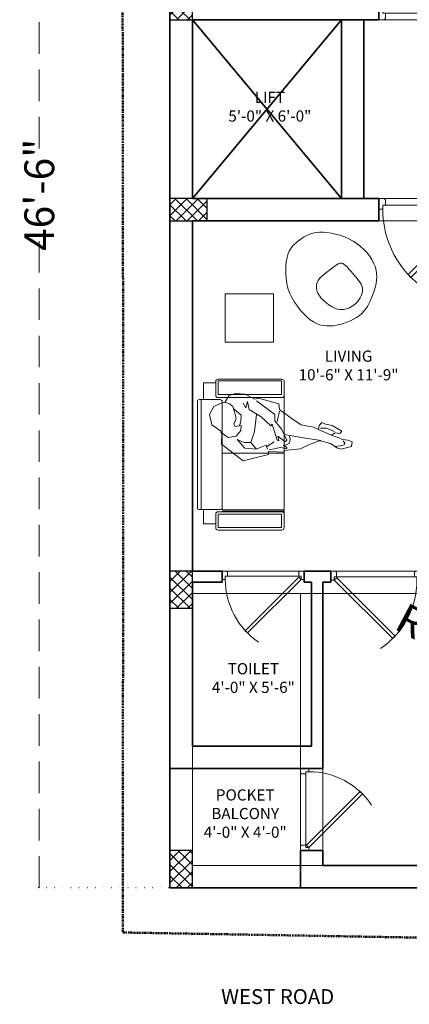
# Model space of a CAD drawing. Units: inches. Extents: x -16911 to -9621, y -48626 to -46270.
# Tile 6 of 20: x -12122 to -11965, y -48264 to -47867. Entities that reach past the tile are written whole.
import ezdxf

# ---------------------------------------------------------------- set-up
doc = ezdxf.new("R2010")
doc.units = ezdxf.units.IN
for name, pattern in [('DASHDOT', [1, 0.5, -0.25, 0, -0.25]), ('DASHED', [19.05, 12.7, -6.35]), ('DOT2', [3.175, 0, -3.175])]:
    doc.linetypes.add(name, pattern=pattern)
for name, color, linetype, lineweight in [('A-ANNO-DIMS', 2, 'Continuous', 13), ('A-ANNO-TEXT', 7, 'Continuous', 18), ('A-AREA-IDEN', 3, 'Continuous', 18), ('A-DOOR', 4, 'Continuous', 18), ('A-FURN', 8, 'Continuous', 13), ('A-WALL', 7, 'Continuous', 35), ('C-PROP', 6, 'DASHDOT', 50), ('column', 12, 'Continuous', 30), ('DOOR', 143, 'Continuous', 9), ('EXT BEAM', 132, 'Continuous', 13), ('furniture', 35, 'Continuous', 15), ('Man', 8, 'Continuous', 5), ('S-BEAM', 132, 'Continuous', 25), ('S-COLS', 1, 'Continuous', 30)]:
    doc.layers.add(name, color=color, linetype=linetype, lineweight=lineweight)
doc.styles.add('style9', font='swisscl.ttf', dxfattribs={"height": 12})
doc.dimstyles.new('Dim9', dxfattribs={"dimtxt": 10, "dimasz": 0.199219, "dimexe": 1, "dimexo": 0.5, "dimgap": 1, "dimtad": 0, "dimdec": 1, "dimzin": 0, "dimdsep": 46, "dimlunit": 4, "dimtxsty": 'style9', "dimblk": 'ARCHTICK', "dimcen": 0.09, "dimclrd": 256, "dimclrt": 256, "dimadec": 0, "dimazin": 0, "dimtfac": 1, "dimtdec": 1, "dimtix": 1, "dimtofl": 0, "dimtmove": 1, "dimatfit": 3, "dimfxl": 9, "dimtolj": 1, "dimtzin": 0, "dimlwd": -1, "dimarcsym": 0})

# ---------------------------------------------------------------- blocks, each defined once
blk = doc.blocks.new('Bipman02')
blk.add_lwpolyline([(0.5871, -0.067), (0.6175, -0.0496), (0.6523, -0.0539), (0.6697, -0.0376), (0.5958, 0.0069), (0.5437, 0.0156), (0.5164, 0.0297), (0.4959, 0.0069), (0.4915, -0.0235), (0.4524, -0.0061), (0.3568, 0.0113), (0.2917, 0.0548), (0.1917, 0.1287), (0.1874, 0.1722), (0.031, 0.2156), (0.0049, 0.2069), (-0.0689, 0.2461), (-0.1471, 0.2504), (-0.1949, 0.233), (-0.2253, 0.1808), (-0.2384, 0.1852), (-0.3079, 0.1504), (-0.3426, 0.0895), (-0.3253, 0.0113), (-0.2558, -0.0365), (-0.2471, -0.0583), (-0.2514, -0.1365), (-0.0863, -0.2626), (0.1092, -0.2148), (0.1092, -0.193), (0.2265, -0.1974), (0.2308, -0.1844), (0.3525, -0.1713), (0.409, -0.1452), (0.4872, -0.1148), (0.5089, -0.1104), (0.5828, -0.1322), (0.6088, -0.1496), (0.6295, -0.1636), (0.661, -0.1757), (0.7435, -0.1539), (0.7478, -0.1191), (0.7143, -0.1051), (0.674, -0.1017), (0.6392, -0.0844)], close=True)
for points in [[(-0.2558, -0.0452), (-0.1993, -0.0844), (-0.1385, -0.0757), (-0.1037, -0.0322), (-0.0994, 0.0069), (-0.1471, -0.0018), (-0.1558, 0.0156), (-0.1385, 0.0591), (-0.1515, 0.1113), (-0.1645, 0.1504), (-0.1906, 0.1722), (-0.2167, 0.1808)], [(-0.0863, 0.1765), (-0.0646, 0.1417), (-0.0516, 0.1895), (-0.0385, 0.1287), (0.0527, 0.0722), (0.1266, 0.0026), (0.1353, 0.0156), (0.1744, -0.1061), (0.1874, -0.1104), (0.1787, -0.0757), (0.2352, -0.1191), (0.2482, -0.1061), (0.2091, -0.0235), (0.157, 0.0417), (0.157, 0.0895), (0.018, 0.1939)], [(-0.1558, 0.133), (-0.0994, 0.0852), (-0.1037, 0.033), (-0.1124, 0.0069)], [(0.018, 0.0895), (0.0006, -0.0409), (-0.0255, -0.1235), (-0.0776, -0.1235), (-0.1298, -0.1017), (-0.0733, -0.167), (0.0136, -0.1757), (0.0918, -0.1452), (0.1005, -0.1757)], [(0.1917, 0.1156), (0.1744, 0.0374)], [(0.2308, -0.0626), (0.3612, -0.0844), (0.5089, -0.1095)], [(0.4915, -0.0235), (0.5871, -0.067)], [(0.5045, -0.0148), (0.5523, -0.0148), (0.6132, -0.0409)], [(-0.0255, -0.1235), (0.0136, -0.1713)], [(0.0962, -0.1539), (0.1526, -0.1191)], [(0.2699, -0.0757), (0.2743, -0.0974), (0.2699, -0.1278), (0.2439, -0.1409), (0.2222, -0.1452), (0.2482, -0.1626), (0.2482, -0.1713), (0.2004, -0.1626), (0.1135, -0.18)], [(0.6783, -0.1104), (0.6914, -0.1278), (0.687, -0.1409), (0.6566, -0.1496), (0.6088, -0.1539)]]:
    blk.add_lwpolyline(points)
blk = doc.blocks.new('erertety')
at = {"layer": 'furniture', "ltscale": 0.2}
for p, q in [((-17662.13, -45230.66), (-17662.13, -45176.69)), ((-17693.83, -45223.2), (-17693.83, -45184.43)), ((-17685.49, -45183.68), (-17693.08, -45183.68)), ((-17684.74, -45223.2), (-17684.74, -45184.43)), ((-17684.74, -45203.31), (-17662.13, -45203.31)), ((-17685.49, -45223.95), (-17693.08, -45223.95)), ((-17691.58, -45223.95), (-17691.58, -45229.1)), ((-17684.74, -45223.99), (-17662.13, -45223.99)), ((-17684.74, -45224.55), (-17662.13, -45224.55)), ((-17684.74, -45224.55), (-17662.13, -45224.55)), ((-17691.58, -45229.1), (-17687.09, -45229.1))]:
    blk.add_line(p, q, dxfattribs=at)
blk.add_lwpolyline([(-17687.09, -45177.54), (-17691.58, -45177.54), (-17691.58, -45183.68)], dxfattribs=at)
for points in [[(-17662.13, -45182.17), (-17662.13, -45176.97, 0.414214), (-17662.87, -45176.22), (-17686.34, -45176.22, 0.414214), (-17687.09, -45176.97), (-17687.09, -45182.17, 0.414214), (-17686.34, -45182.91), (-17662.87, -45182.91, 0.414214)], [(-17662.13, -45225.47), (-17662.13, -45230.66, -0.414214), (-17662.87, -45231.41), (-17686.34, -45231.41, -0.414214), (-17687.09, -45230.66), (-17687.09, -45225.47, -0.414214), (-17686.34, -45224.72), (-17662.87, -45224.72, -0.414214)]]:
    blk.add_lwpolyline(points, format="xyb", close=True, dxfattribs=at)
for points in [[(-17663.01, -45181.75), (-17663.01, -45176.82), (-17686.21, -45176.82), (-17686.21, -45181.75)], [(-17692.4, -45183.68), (-17692.4, -45223.95), (-17692.4, -45223.95), (-17692.4, -45183.68)], [(-17663.01, -45225.6), (-17663.01, -45230.53), (-17686.21, -45230.53), (-17686.21, -45225.6)]]:
    blk.add_lwpolyline(points, close=True, dxfattribs=at)
for centre, start, end in [((-17693.08, -45184.43), 90, 180), ((-17685.49, -45184.43), 0, 90), ((-17693.08, -45223.2), 180, 270), ((-17685.49, -45223.2), 270, 0)]:
    blk.add_arc(centre, 0.748, start, end, dxfattribs=at)
at = {"layer": 'furniture', "ltscale": 0.2, "xscale": 47.90818138957024, "yscale": 47.90818138957024, "zscale": 47.90818138957024}
blk.add_blockref('Bipman02', (-17673, -45193.44, 0), dxfattribs=at)
blk = doc.blocks.new('rthrty')
at = {"layer": 'furniture'}
blk.add_open_spline([(-17650.3, -45154.53), (-17651.97, -45142.9), (-17645.3, -45136.31), (-17637.11, -45132.37), (-17620.71, -45137.17), (-17612.47, -45149.45), (-17615.73, -45159.71), (-17619.67, -45168.02), (-17632.28, -45172.65), (-17641.84, -45170.43), (-17649.5, -45159.42), (-17650.3, -45154.53)], degree=3, dxfattribs=at)
at = {"layer": 'Man'}
blk.add_open_spline([(-17632.99, -45149.02), (-17629.89, -45146.6), (-17628, -45145.12), (-17623.29, -45151.15), (-17618.06, -45156.77), (-17623.15, -45164.08), (-17628.28, -45165.32), (-17631.61, -45164.6), (-17638.01, -45159.61), (-17638.81, -45154.69), (-17636.9, -45151.81), (-17632.99, -45149.02), (-17632.99, -45149.02)], degree=3, dxfattribs=at)
blk = doc.blocks.new('A$C1C9D3E54')
at = {"layer": 'DOOR'}
blk.add_line((18676.53, 5780.72), (18710.53, 5780.72), dxfattribs=at)
blk.add_lwpolyline([(18685.01, 5806.62), (18710.47, 5781.16), (18711.53, 5782.22), (18686.07, 5807.68), (18685.01, 5806.62)], dxfattribs=at)
blk.add_lwpolyline([(18674.03, 5778.22), (18676.03, 5778.22), (18674.03, 5778.22), (18674.03, 5782.22), (18675.53, 5782.22), (18675.53, 5780.72), (18676.53, 5780.72), (18676.53, 5778.72), (18676.41, 5778.72), (18676.41, 5778.6, -0.414214), (18676.16, 5778.35), (18676.03, 5778.35), (18676.03, 5778.22)], format="xyb", dxfattribs=at)
blk.add_lwpolyline([(18713.03, 5782.22), (18711.53, 5782.22), (18711.53, 5780.72), (18710.53, 5780.72), (18710.53, 5778.72), (18710.66, 5778.72), (18710.66, 5778.6, 0.414214), (18710.91, 5778.35), (18711.03, 5778.35), (18711.03, 5778.22), (18713.03, 5778.22), (18711.03, 5778.22), (18713.03, 5778.22), (18713.03, 5782.22)], format="xyb", close=True, dxfattribs=at)
blk.add_arc((18711.53, 5782.22), 36, 124.0336, 180, dxfattribs=at)
blk = doc.blocks.new('COLUMNS')
at = {"layer": 'column'}
h = blk.add_hatch(dxfattribs=at)
h.set_pattern_fill('ANSI37', color=256, angle=-900)
h.set_pattern_definition([(225, (-45817.4075, 11499.4594), (2.24506403, -2.24506403), []), (315, (-45817.4075, 11499.4594), (2.24506403, 2.24506403), [])])
h.paths.add_polyline_path([(-12052.47, -46580.36), (-12061.47, -46580.36), (-12061.47, -46595.36), (-12052.47, -46595.36)])
h = blk.add_hatch(dxfattribs=at)
h.set_pattern_fill('ANSI37', color=256, angle=-810)
h.set_pattern_definition([(315, (-70141.2892, -80432.2886), (2.24506403, 2.24506403), []), (45, (-70141.2892, -80432.2886), (-2.24506403, 2.24506403), [])])
h.paths.add_polyline_path([(-12061.47, -46667.36), (-12061.47, -46676.36), (-12046.47, -46676.36), (-12046.47, -46667.36)])
h = blk.add_hatch(dxfattribs=at)
h.set_pattern_fill('ANSI37', color=256, angle=-540)
h.set_pattern_definition([(225, (-45817.4075, 11262.5055), (2.24506403, -2.24506403), []), (315, (-45817.4075, 11262.5055), (2.24506403, 2.24506403), [])])
h.paths.add_polyline_path([(-12052.47, -46817.31), (-12061.47, -46817.31), (-12061.47, -46832.31), (-12052.47, -46832.31)])
h = blk.add_hatch(dxfattribs=at)
h.set_pattern_fill('ANSI37', color=256, angle=-720)
h.set_pattern_definition([(45, (21703.4588, -105024.6242), (-2.24506403, 2.24506403), []), (135, (21703.4588, -105024.6242), (-2.24506403, -2.24506403), [])])
h.paths.add_polyline_path([(-12061.47, -46944.81), (-12052.47, -46944.81), (-12052.47, -46929.81), (-12061.47, -46929.81)])
at = {"layer": 'column', "ltscale": 0.05}
for points in [[(-12061.47, -46595.36), (-12052.47, -46595.36), (-12052.47, -46580.36), (-12061.47, -46580.36)], [(-12046.47, -46676.36), (-12046.47, -46667.36), (-12061.47, -46667.36), (-12061.47, -46676.36)], [(-12061.47, -46832.31), (-12052.47, -46832.31), (-12052.47, -46817.31), (-12061.47, -46817.31)], [(-12052.47, -46929.81), (-12061.47, -46929.81), (-12061.47, -46944.81), (-12052.47, -46944.81)]]:
    blk.add_lwpolyline(points, close=True, dxfattribs=at)
blk = doc.blocks.new('TYPICAL BEAMS G-2')
at = {"layer": 'EXT BEAM'}
for p, q in [((-12061.47, -48216.7), (-12061.47, -47658.74)), ((-12052.47, -47939.24), (-12052.47, -47667.74)), ((-12052.47, -47867.24), (-11924.72, -47867.24)), ((-11992.47, -47867.24), (-11992.47, -47939.24)), ((-11983.47, -47867.24), (-11983.47, -47939.24)), ((-12046.47, -47939.24), (-11929.47, -47939.24)), ((-12052.47, -48089.2), (-12052.47, -47948.24)), ((-12046.47, -47948.24), (-11929.47, -47948.24)), ((-12052.47, -48089.2), (-11747.92, -48089.2)), ((-12052.47, -48216.7), (-12052.47, -48098.2)), ((-12052.47, -48098.2), (-11879.72, -48098.2)), ((-12008.97, -48098.2), (-12008.97, -48207.7)), ((-11999.97, -48098.2), (-11999.97, -48207.7)), ((-12052.47, -48207.7), (-11879.72, -48207.7)), ((-12061.47, -48216.7), (-11738.92, -48216.7))]:
    blk.add_line(p, q, dxfattribs=at)
blk = doc.blocks.new('_ArchTick')
at = {"color": 0, "linetype": 'ByBlock', "const_width": 0.15}
blk.add_lwpolyline([(-0.5, -0.5), (0.5, 0.5)], dxfattribs=at)
blk = doc.blocks.new('*D132')
at = {"layer": 'A-ANNO-DIMS', "color": 0, "linetype": 'DOT2', "lineweight": -2, "transparency": 16777216}
for p, q in [((-12061.97, -47658.74), (-12115.09, -47658.74)), ((-12061.97, -48216.7), (-12115.09, -48216.7))]:
    blk.add_line(p, q, dxfattribs=at)
at = {"layer": 'A-ANNO-DIMS', "linetype": 'DASHED', "transparency": 16777216}
for p, q in [((-12114.09, -47658.74), (-12114.09, -47920.08)), ((-12114.09, -48216.7), (-12114.09, -47955.35))]:
    blk.add_line(p, q, dxfattribs=at)
at = {"layer": 'Defpoints', "color": 0, "transparency": 16777216}
for p in [(-12061.47, -47658.74), (-12114.09, -48216.7), (-12061.47, -48216.7)]:
    blk.add_point(p, dxfattribs=at)
at = {"layer": 'A-ANNO-DIMS', "transparency": 16777216, "xscale": 0.19921875, "yscale": 0.19921875, "zscale": 0.19921875}
for p, rotation in [((-12114.09, -47658.74), 90), ((-12114.09, -48216.7), 270)]:
    blk.add_blockref('_ArchTick', p, dxfattribs=dict(at, rotation=rotation))
at = {"layer": 'A-ANNO-DIMS', "transparency": 16777216, "insert": (-12114.09, -47937.72), "char_height": 12, "attachment_point": 5, "rotation": 90, "style": 'style9'}
blk.add_mtext('\\A1;46\'-6"', dxfattribs=at)
blk = doc.blocks.new('*D136')
at = {"layer": 'A-ANNO-DIMS', "color": 0, "lineweight": -2, "transparency": 16777216}
for p, q in [((-11995.43, -48092.88), (-11995.25, -48092.88)), ((-11995.34, -48092.97), (-11995.34, -48092.79))]:
    blk.add_line(p, q, dxfattribs=at)
at = {"layer": 'A-ANNO-DIMS', "linetype": 'DASHED', "transparency": 16777216}
blk.add_line((-11964.07, -48109.5), (-11965.99, -48108.48), dxfattribs=at)
at = {"layer": 'Defpoints', "color": 0, "transparency": 16777216}
for p in [(-11995.34, -48092.88), (-11965.99, -48108.48)]:
    blk.add_point(p, dxfattribs=at)
at = {"layer": 'A-ANNO-DIMS', "transparency": 16777216, "xscale": 0.19921875, "yscale": 0.19921875, "zscale": 0.19921875, "rotation": 152.0167210822722}
blk.add_blockref('_ArchTick', (-11965.99, -48108.48), dxfattribs=at)
at = {"layer": 'A-ANNO-DIMS', "transparency": 16777216, "insert": (-11948.39, -48117.83), "char_height": 12, "attachment_point": 5, "rotation": 332.0167, "style": 'style9'}
blk.add_mtext('\\A1;R2\'-9"', dxfattribs=at)

msp = doc.modelspace()

# ---------------------------------------------------------------- linework, layer by layer
at = {"layer": 'A-FURN'}
msp.add_lwpolyline([(-12019.878, -47977.637), (-12039.238, -47977.637), (-12039.238, -47996.997), (-12019.878, -47996.997)], close=True, dxfattribs=at)
at = {"layer": 'A-WALL'}
for p, q in [((-12061.474, -48168.696), (-12061.474, -47706.742)), ((-11977.474, -47867.242), (-11977.474, -47858.242)), ((-12052.474, -47939.242), (-12052.474, -47867.242)), ((-11977.474, -47867.242), (-12052.474, -47867.242)), ((-12052.474, -47867.242), (-11992.474, -47939.242)), ((-12052.474, -47939.242), (-11992.474, -47867.242)), ((-11992.474, -47939.242), (-11992.474, -47867.242)), ((-11983.474, -47939.242), (-11983.474, -47867.242)), ((-11977.474, -47939.242), (-12052.474, -47939.242)), ((-11977.474, -47948.242), (-11977.474, -47939.242)), ((-12052.474, -48089.196), (-12052.474, -47948.242)), ((-11977.474, -47948.242), (-12052.474, -47948.242)), ((-12052.474, -48089.196), (-12040.474, -48089.196)), ((-12040.474, -48089.196), (-12040.474, -48093.696)), ((-12007.474, -48089.196), (-11996.724, -48089.196)), ((-12007.474, -48089.196), (-12007.474, -48093.696)), ((-11996.724, -48093.696), (-11996.724, -48089.196)), ((-12052.474, -48159.696), (-12052.474, -48093.696)), ((-12052.474, -48093.696), (-12040.474, -48093.696)), ((-12007.474, -48093.696), (-12004.474, -48093.696)), ((-12004.474, -48159.696), (-12004.474, -48093.696)), ((-11999.974, -48168.696), (-11999.974, -48093.696)), ((-11999.974, -48093.696), (-11996.724, -48093.696)), ((-12052.474, -48159.696), (-12004.474, -48159.696)), ((-12061.474, -48216.696), (-12061.474, -48168.696)), ((-12061.474, -48168.696), (-11999.974, -48168.696)), ((-12008.974, -48216.696), (-12008.974, -48201.696)), ((-12008.974, -48201.696), (-11999.974, -48201.696)), ((-11999.974, -48207.696), (-11999.974, -48201.696)), ((-11999.974, -48207.696), (-11879.724, -48207.696)), ((-12061.474, -48216.696), (-12008.974, -48216.696)), ((-12008.974, -48216.696), (-11738.925, -48216.696))]:
    msp.add_line(p, q, dxfattribs=at)
at = {"layer": 'C-PROP'}
msp.add_lwpolyline([(-12080.474, -48234.696), (-11720.293, -48240.921), (-11719.732, -48212.333), (-11720.395, -48127.492), (-11721.561, -47881.398), (-11721.175, -47639.742), (-12080.838, -47634.697), (-12080.3, -48034.841)], close=True, dxfattribs=at)

# ---------------------------------------------------------------- block references
at = {"layer": 'A-DOOR', "xscale": 1.076923076922859, "yscale": 1.076923076922859, "zscale": 1.076923076922859}
msp.add_blockref('A$C1C9D3E54', (-32087.969, -54089.945), dxfattribs=at)
at = {"layer": 'A-DOOR'}
for p, xscale, yscale, zscale, rotation in [((-32087.969, -41716.539), -1.076923076922859, 1.076923076922859, 1.076923076922859, 180), ((-27841.577, -43199.929), -0.8461538461538624, 0.8461538461538624, 0.8461538461538624, 180), ((5276.842, -42755.451), 0.9230769230769229, 0.9230769230769229, 0.9230769230769229, 180), ((-16898.241, -32367.593), 0.8461538461538624, 0.8461538461538624, 0.8461538461538624, 270)]:
    msp.add_blockref('A$C1C9D3E54', p, dxfattribs=dict(at, xscale=xscale, yscale=yscale, zscale=zscale, rotation=rotation))
at = {"layer": 'A-FURN'}
msp.add_blockref('rthrty', (5635.852, -2818.939), dxfattribs=at)
at = {"layer": 'A-FURN', "xscale": 1.1, "yscale": 1.1, "zscale": 1.1}
msp.add_blockref('erertety', (7412.76, 1681.863, 0), dxfattribs=at)
at = {"layer": 'S-BEAM'}
msp.add_blockref('TYPICAL BEAMS G-2', (0, 0), dxfattribs=at)
at = {"layer": 'S-COLS'}
msp.add_blockref('COLUMNS', (0, -1271.886), dxfattribs=at)

# ---------------------------------------------------------------- texts
at = {"layer": 'A-ANNO-TEXT', "ltscale": 10, "insert": (-12040.885, -48257.497), "char_height": 6, "width": 70.69764, "attachment_point": 1, "style": 'style9'}
msp.add_mtext('\\A1;{\\fCentury Gothic|b0|i0|c0|p34;WEST ROAD}', dxfattribs=at)
at = {"layer": 'A-AREA-IDEN', "ltscale": 10, "char_height": 4.5, "width": 42.823, "attachment_point": 1, "style": 'style9'}
for s, insert in [('\\A1;\\pxqc;{\\fCentury Gothic|b0|i0|c0|p34;LIFT\\P5\'-0" X 6\'-0"}', (-12042.698, -47896.277)), ('\\A1;\\pxqc;{\\fCentury Gothic|b0|i0|c0|p34;LIVING\\P10\'-6" X 11\'-9"}', (-12011.012, -48000.428)), ('\\A1;\\pxqc;{\\fCentury Gothic|b0|i0|c0|p34;TOILET\\P4\'-0" X 5\'-6"}', (-12049.33, -48126.259)), ('\\A1;\\pxqc;{\\fCentury Gothic|b0|i0|c0|p34;POCKET BALCONY\\P4\'-0" X 4\'-0"}', (-12052.615, -48177.063))]:
    msp.add_mtext(s, dxfattribs=dict(at, insert=insert))

# ---------------------------------------------------------------- dimensions: what is measured, and where the dimension line sits
at = {"layer": 'A-ANNO-DIMS'}
dim = msp.add_linear_dim(base=(-12114.088, -48216.696), p1=(-12061.474, -47658.742), p2=(-12061.474, -48216.696), angle=90, dimstyle='Dim9', override={"dimdec": 1, "dimlfac": 1, "dimrnd": 0, "dimzin": 1, "dimdsep": 46, "dimlunit": 4, "dimfrac": 2}, dxfattribs=at)
dim.commit()
dim.dimension.update_dxf_attribs({"geometry": '*D132', "text_midpoint": (-12114.088, -47937.719)})
dim = msp.add_radius_dim(center=(-11995.34, -48092.885), mpoint=(-11965.994, -48108.477), dimstyle='Dim9', override={"dimdec": 1, "dimlfac": 1, "dimrnd": 0, "dimzin": 1, "dimdsep": 46, "dimlunit": 4, "dimfrac": 2}, dxfattribs=at)
dim.commit()
dim.dimension.update_dxf_attribs({"geometry": '*D136', "text_midpoint": (-11948.387, -48117.832), "dimtype": 164})

doc.saveas('drawing.dxf')
